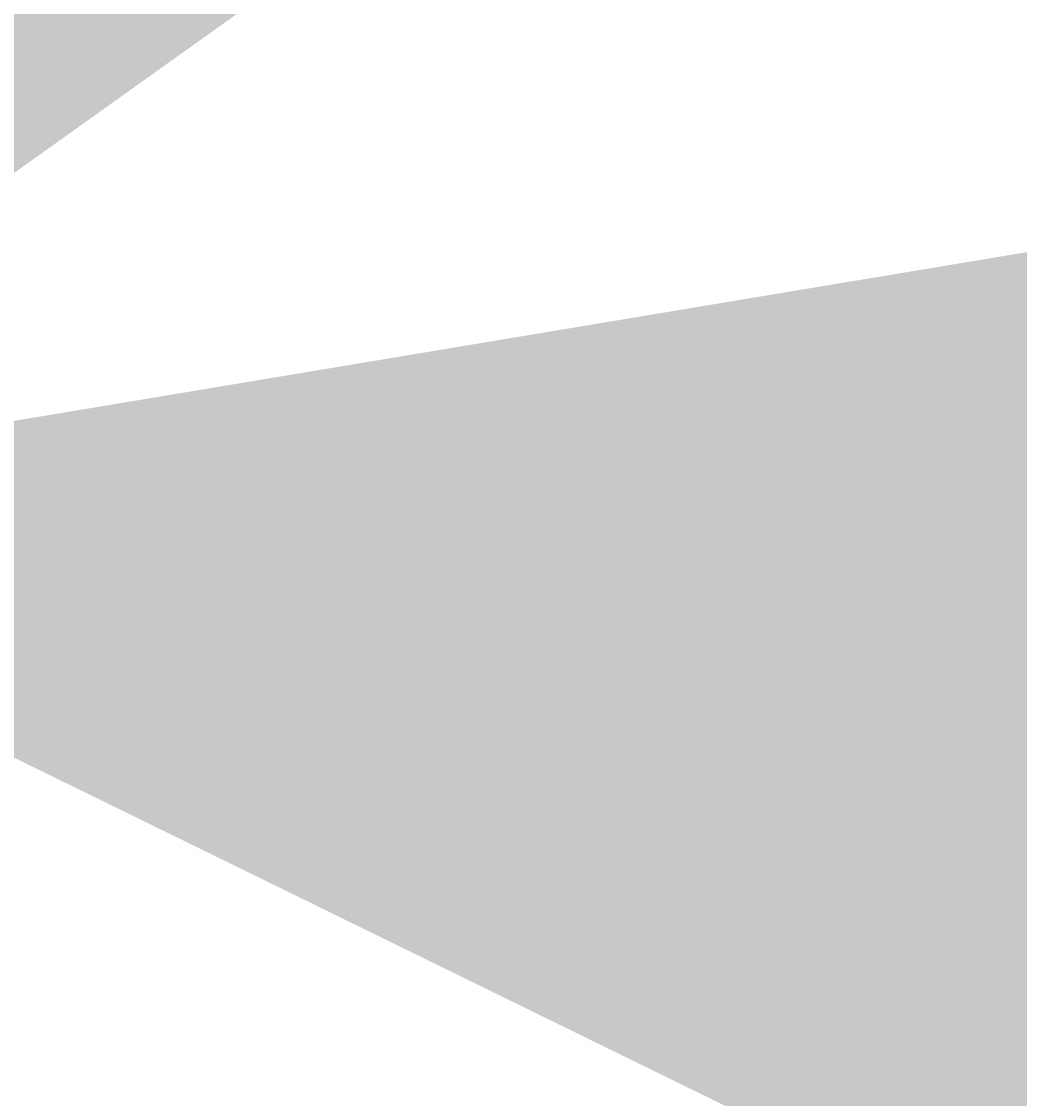
# Model space of a CAD drawing. Units: millimetres. Extents: x -22994 to 29398, y -19990 to 20176.
# Tile 131 of 135: x 2052 to 5745, y -1986 to 2002. Entities that reach past the tile are written whole.
import ezdxf

# ---------------------------------------------------------------- set-up
doc = ezdxf.new("R2010")
doc.units = ezdxf.units.MM
doc.header["$MEASUREMENT"] = 0
doc.layers.add('M-DIMS', color=2, linetype='Continuous', lineweight=18)
doc.styles.get("Standard").update_dxf_attribs({"font": 'arial.ttf'})
doc.dimstyles.get("Standard").update_dxf_attribs({"dimtxt": 0.18, "dimasz": 10000, "dimexe": 0.18, "dimexo": 0.0625, "dimgap": 0.09, "dimtad": 0, "dimtih": 1, "dimtoh": 1, "dimdec": 0, "dimzin": 0, "dimdsep": 46, "dimtxsty": 'Standard', "dimcen": 0.09, "dimadec": 0, "dimazin": 0, "dimtfac": 1, "dimtdec": 0, "dimtofl": 0, "dimtmove": 0, "dimatfit": 3, "dimfxl": 1, "dimtolj": 1, "dimtzin": 0, "dimlwd": 30, "dimarcsym": 0})

# ---------------------------------------------------------------- blocks, each defined once
blk = doc.blocks.new('*D2')
at = {"layer": 'Defpoints', "color": 0, "transparency": 16777216}
for p in [(6.7, 10.3), (290.9, 10.3), (290.9, -5.1)]:
    blk.add_point(p, dxfattribs=at)
at = {"layer": 'M-DIMS', "color": 0, "lineweight": -2, "transparency": 16777216}
for p, q in [((6.7, 10.2), (6.7, -5.3)), ((290.9, 10.2), (290.9, -5.3))]:
    blk.add_line(p, q, dxfattribs=at)
at = {"layer": 'M-DIMS', "color": 0, "lineweight": 30, "transparency": 16777216}
for p, q in [((-9993.3, -5.1), (-19993.3, -5.1)), ((10290.9, -5.1), (20290.9, -5.1))]:
    blk.add_line(p, q, dxfattribs=at)
at = {"layer": 'M-DIMS', "color": 0, "transparency": 16777216}
for points in [[(-9993.3, 1661.6), (-9993.3, -1671.7), (6.7, -5.1)], [(10290.9, 1661.6), (10290.9, -1671.7), (290.9, -5.1)]]:
    blk.add_solid(points, dxfattribs=at)
at = {"layer": 'M-DIMS', "color": 0, "transparency": 16777216, "insert": (148.8, -5.1), "char_height": 0.18, "attachment_point": 5}
blk.add_mtext('\\A1;284.2', dxfattribs=at)
blk = doc.blocks.new('*D3')
at = {"layer": 'Defpoints', "color": 0, "transparency": 16777216}
for p in [(110.3, 204.2), (110.3, 176.4), (95.8, 128)]:
    blk.add_point(p, dxfattribs=at)
at = {"layer": 'M-DIMS', "color": 0, "lineweight": 30, "transparency": 16777216}
for p, q in [((-9904.2, 204.2), (-19904.2, 204.2)), ((10110.3, 204.2), (20110.3, 204.2))]:
    blk.add_line(p, q, dxfattribs=at)
at = {"layer": 'M-DIMS', "color": 0, "lineweight": -2, "transparency": 16777216}
for p, q in [((95.8, 128), (95.8, 204.3)), ((110.3, 176.4), (110.3, 204.3))]:
    blk.add_line(p, q, dxfattribs=at)
at = {"layer": 'M-DIMS', "color": 0, "transparency": 16777216}
for points in [[(-9904.2, 1870.8), (-9904.2, -1462.5), (95.8, 204.2)], [(10110.3, 1870.8), (10110.3, -1462.5), (110.3, 204.2)]]:
    blk.add_solid(points, dxfattribs=at)
at = {"layer": 'M-DIMS', "color": 0, "transparency": 16777216, "insert": (103, 204.2), "char_height": 0.18, "attachment_point": 5}
blk.add_mtext('\\A1;14.432', dxfattribs=at)
blk = doc.blocks.new('*D4')
at = {"layer": 'Defpoints', "color": 0, "transparency": 16777216}
for p in [(116.3, 204.2), (110.3, 176.4), (116.3, 176.4)]:
    blk.add_point(p, dxfattribs=at)
at = {"layer": 'M-DIMS', "color": 0, "lineweight": 30, "transparency": 16777216}
for p, q in [((-9889.7, 204.2), (-19889.7, 204.2)), ((10116.3, 204.2), (20116.3, 204.2))]:
    blk.add_line(p, q, dxfattribs=at)
at = {"layer": 'M-DIMS', "color": 0, "lineweight": -2, "transparency": 16777216}
for p, q in [((110.3, 176.4), (110.3, 204.3)), ((116.3, 176.4), (116.3, 204.3))]:
    blk.add_line(p, q, dxfattribs=at)
at = {"layer": 'M-DIMS', "color": 0, "transparency": 16777216}
for points in [[(-9889.7, 1870.8), (-9889.7, -1462.5), (110.3, 204.2)], [(10116.3, 1870.8), (10116.3, -1462.5), (116.3, 204.2)]]:
    blk.add_solid(points, dxfattribs=at)
at = {"layer": 'M-DIMS', "color": 0, "transparency": 16777216, "insert": (113.3, 204.2), "char_height": 0.18, "attachment_point": 5}
blk.add_mtext('\\A1;6', dxfattribs=at)
blk = doc.blocks.new('*D5')
at = {"layer": 'Defpoints', "color": 0, "transparency": 16777216}
for p in [(181.3, 204.2), (116.3, 176.4), (181.3, 176.4)]:
    blk.add_point(p, dxfattribs=at)
at = {"layer": 'M-DIMS', "color": 0, "lineweight": 30, "transparency": 16777216}
for p, q in [((-9883.7, 204.2), (-19883.7, 204.2)), ((10181.3, 204.2), (20181.3, 204.2))]:
    blk.add_line(p, q, dxfattribs=at)
at = {"layer": 'M-DIMS', "color": 0, "lineweight": -2, "transparency": 16777216}
for p, q in [((116.3, 176.4), (116.3, 204.3)), ((181.3, 176.4), (181.3, 204.3))]:
    blk.add_line(p, q, dxfattribs=at)
at = {"layer": 'M-DIMS', "color": 0, "transparency": 16777216}
for points in [[(-9883.7, 1870.8), (-9883.7, -1462.5), (116.3, 204.2)], [(10181.3, 1870.8), (10181.3, -1462.5), (181.3, 204.2)]]:
    blk.add_solid(points, dxfattribs=at)
at = {"layer": 'M-DIMS', "color": 0, "transparency": 16777216, "insert": (148.8, 204.2), "char_height": 0.18, "attachment_point": 5}
blk.add_mtext('\\A1;65', dxfattribs=at)
blk = doc.blocks.new('*D6')
at = {"layer": 'Defpoints', "color": 0, "transparency": 16777216}
for p in [(187.3, 204.2), (181.3, 176.4), (187.3, 176.4)]:
    blk.add_point(p, dxfattribs=at)
at = {"layer": 'M-DIMS', "color": 0, "lineweight": 30, "transparency": 16777216}
for p, q in [((-9818.7, 204.2), (-19818.7, 204.2)), ((10187.3, 204.2), (20187.3, 204.2))]:
    blk.add_line(p, q, dxfattribs=at)
at = {"layer": 'M-DIMS', "color": 0, "lineweight": -2, "transparency": 16777216}
for p, q in [((181.3, 176.4), (181.3, 204.3)), ((187.3, 176.4), (187.3, 204.3))]:
    blk.add_line(p, q, dxfattribs=at)
at = {"layer": 'M-DIMS', "color": 0, "transparency": 16777216}
for points in [[(-9818.7, 1870.8), (-9818.7, -1462.5), (181.3, 204.2)], [(10187.3, 1870.8), (10187.3, -1462.5), (187.3, 204.2)]]:
    blk.add_solid(points, dxfattribs=at)
at = {"layer": 'M-DIMS', "color": 0, "transparency": 16777216, "insert": (184.3, 204.2), "char_height": 0.18, "attachment_point": 5}
blk.add_mtext('\\A1;6', dxfattribs=at)
blk = doc.blocks.new('*D7')
at = {"layer": 'Defpoints', "color": 0, "transparency": 16777216}
for p in [(201.7, 204.2), (187.3, 176.4), (201.7, 128)]:
    blk.add_point(p, dxfattribs=at)
at = {"layer": 'M-DIMS', "color": 0, "lineweight": 30, "transparency": 16777216}
for p, q in [((-9812.7, 204.2), (-19812.7, 204.2)), ((10201.7, 204.2), (20201.7, 204.2))]:
    blk.add_line(p, q, dxfattribs=at)
at = {"layer": 'M-DIMS', "color": 0, "lineweight": -2, "transparency": 16777216}
for p, q in [((187.3, 176.4), (187.3, 204.3)), ((201.7, 128), (201.7, 204.3))]:
    blk.add_line(p, q, dxfattribs=at)
at = {"layer": 'M-DIMS', "color": 0, "transparency": 16777216}
for points in [[(-9812.7, 1870.8), (-9812.7, -1462.5), (187.3, 204.2)], [(10201.7, 1870.8), (10201.7, -1462.5), (201.7, 204.2)]]:
    blk.add_solid(points, dxfattribs=at)
at = {"layer": 'M-DIMS', "color": 0, "transparency": 16777216, "insert": (194.5, 204.2), "char_height": 0.18, "attachment_point": 5}
blk.add_mtext('\\A1;14.432', dxfattribs=at)
blk = doc.blocks.new('*D8')
at = {"layer": 'Defpoints', "color": 0, "transparency": 16777216}
for p in [(227.6, 204.2), (201.7, 128), (227.6, 146.7)]:
    blk.add_point(p, dxfattribs=at)
at = {"layer": 'M-DIMS', "color": 0, "lineweight": 30, "transparency": 16777216}
for p, q in [((-9798.3, 204.2), (-19798.3, 204.2)), ((10227.6, 204.2), (20227.6, 204.2))]:
    blk.add_line(p, q, dxfattribs=at)
at = {"layer": 'M-DIMS', "color": 0, "lineweight": -2, "transparency": 16777216}
for p, q in [((201.7, 128), (201.7, 204.3)), ((227.6, 146.8), (227.6, 204.3))]:
    blk.add_line(p, q, dxfattribs=at)
at = {"layer": 'M-DIMS', "color": 0, "transparency": 16777216}
for points in [[(-9798.3, 1870.8), (-9798.3, -1462.5), (201.7, 204.2)], [(10227.6, 1870.8), (10227.6, -1462.5), (227.6, 204.2)]]:
    blk.add_solid(points, dxfattribs=at)
at = {"layer": 'M-DIMS', "color": 0, "transparency": 16777216, "insert": (214.7, 204.2), "char_height": 0.18, "attachment_point": 5}
blk.add_mtext('\\A1;25.95', dxfattribs=at)
blk = doc.blocks.new('*D10')
at = {"layer": 'Defpoints', "color": 0, "transparency": 16777216}
for p in [(125.6, 136.1), (133.3, 136.1), (133.3, -5.1)]:
    blk.add_point(p, dxfattribs=at)
at = {"layer": 'M-DIMS', "color": 0, "lineweight": -2, "transparency": 16777216}
for p, q in [((125.6, 136), (125.6, -5.3)), ((133.3, 136), (133.3, -5.3))]:
    blk.add_line(p, q, dxfattribs=at)
at = {"layer": 'M-DIMS', "color": 0, "lineweight": 30, "transparency": 16777216}
for p, q in [((-9874.4, -5.1), (-19874.4, -5.1)), ((10133.3, -5.1), (20133.3, -5.1))]:
    blk.add_line(p, q, dxfattribs=at)
at = {"layer": 'M-DIMS', "color": 0, "transparency": 16777216}
for points in [[(-9874.4, 1661.6), (-9874.4, -1671.7), (125.6, -5.1)], [(10133.3, 1661.6), (10133.3, -1671.7), (133.3, -5.1)]]:
    blk.add_solid(points, dxfattribs=at)
at = {"layer": 'M-DIMS', "color": 0, "transparency": 16777216, "insert": (129.5, -5.1), "char_height": 0.18, "attachment_point": 5}
blk.add_mtext('\\A1;7.696', dxfattribs=at)
blk = doc.blocks.new('*D11')
at = {"layer": 'Defpoints', "color": 0, "transparency": 16777216}
for p in [(133.3, 136.1), (135.6, 136.1), (135.6, -5.1)]:
    blk.add_point(p, dxfattribs=at)
at = {"layer": 'M-DIMS', "color": 0, "lineweight": -2, "transparency": 16777216}
for p, q in [((133.3, 136), (133.3, -5.3)), ((135.6, 136), (135.6, -5.3))]:
    blk.add_line(p, q, dxfattribs=at)
at = {"layer": 'M-DIMS', "color": 0, "lineweight": 30, "transparency": 16777216}
for p, q in [((-9866.7, -5.1), (-19866.7, -5.1)), ((10135.6, -5.1), (20135.6, -5.1))]:
    blk.add_line(p, q, dxfattribs=at)
at = {"layer": 'M-DIMS', "color": 0, "transparency": 16777216}
for points in [[(-9866.7, 1661.6), (-9866.7, -1671.7), (133.3, -5.1)], [(10135.6, 1661.6), (10135.6, -1671.7), (135.6, -5.1)]]:
    blk.add_solid(points, dxfattribs=at)
at = {"layer": 'M-DIMS', "color": 0, "transparency": 16777216, "insert": (134.5, -5.1), "char_height": 0.18, "attachment_point": 5}
blk.add_mtext('\\A1;2.304', dxfattribs=at)
blk = doc.blocks.new('*D12')
at = {"layer": 'Defpoints', "color": 0, "transparency": 16777216}
for p in [(135.6, 136.1), (145.6, 136.1), (145.6, -5.1)]:
    blk.add_point(p, dxfattribs=at)
at = {"layer": 'M-DIMS', "color": 0, "lineweight": -2, "transparency": 16777216}
for p, q in [((135.6, 136), (135.6, -5.3)), ((145.6, 136), (145.6, -5.3))]:
    blk.add_line(p, q, dxfattribs=at)
at = {"layer": 'M-DIMS', "color": 0, "lineweight": 30, "transparency": 16777216}
for p, q in [((-9864.4, -5.1), (-19864.4, -5.1)), ((10145.6, -5.1), (20145.6, -5.1))]:
    blk.add_line(p, q, dxfattribs=at)
at = {"layer": 'M-DIMS', "color": 0, "transparency": 16777216}
for points in [[(-9864.4, 1661.6), (-9864.4, -1671.7), (135.6, -5.1)], [(10145.6, 1661.6), (10145.6, -1671.7), (145.6, -5.1)]]:
    blk.add_solid(points, dxfattribs=at)
at = {"layer": 'M-DIMS', "color": 0, "transparency": 16777216, "insert": (140.6, -5.1), "char_height": 0.18, "attachment_point": 5}
blk.add_mtext('\\A1;10', dxfattribs=at)
blk = doc.blocks.new('*D13')
at = {"layer": 'Defpoints', "color": 0, "transparency": 16777216}
for p in [(145.6, 136.1), (155.6, 136.1), (155.6, -5.1)]:
    blk.add_point(p, dxfattribs=at)
at = {"layer": 'M-DIMS', "color": 0, "lineweight": -2, "transparency": 16777216}
for p, q in [((145.6, 136), (145.6, -5.3)), ((155.6, 136), (155.6, -5.3))]:
    blk.add_line(p, q, dxfattribs=at)
at = {"layer": 'M-DIMS', "color": 0, "lineweight": 30, "transparency": 16777216}
for p, q in [((-9854.4, -5.1), (-19854.4, -5.1)), ((10155.6, -5.1), (20155.6, -5.1))]:
    blk.add_line(p, q, dxfattribs=at)
at = {"layer": 'M-DIMS', "color": 0, "transparency": 16777216}
for points in [[(-9854.4, 1661.6), (-9854.4, -1671.7), (145.6, -5.1)], [(10155.6, 1661.6), (10155.6, -1671.7), (155.6, -5.1)]]:
    blk.add_solid(points, dxfattribs=at)
at = {"layer": 'M-DIMS', "color": 0, "transparency": 16777216, "insert": (150.6, -5.1), "char_height": 0.18, "attachment_point": 5}
blk.add_mtext('\\A1;10', dxfattribs=at)
blk = doc.blocks.new('*D14')
at = {"layer": 'Defpoints', "color": 0, "transparency": 16777216}
for p in [(155.6, 136.1), (165.6, 136.1), (165.6, -5.1)]:
    blk.add_point(p, dxfattribs=at)
at = {"layer": 'M-DIMS', "color": 0, "lineweight": -2, "transparency": 16777216}
for p, q in [((155.6, 136), (155.6, -5.3)), ((165.6, 136), (165.6, -5.3))]:
    blk.add_line(p, q, dxfattribs=at)
at = {"layer": 'M-DIMS', "color": 0, "lineweight": 30, "transparency": 16777216}
for p, q in [((-9844.4, -5.1), (-19844.4, -5.1)), ((10165.6, -5.1), (20165.6, -5.1))]:
    blk.add_line(p, q, dxfattribs=at)
at = {"layer": 'M-DIMS', "color": 0, "transparency": 16777216}
for points in [[(-9844.4, 1661.6), (-9844.4, -1671.7), (155.6, -5.1)], [(10165.6, 1661.6), (10165.6, -1671.7), (165.6, -5.1)]]:
    blk.add_solid(points, dxfattribs=at)
at = {"layer": 'M-DIMS', "color": 0, "transparency": 16777216, "insert": (160.6, -5.1), "char_height": 0.18, "attachment_point": 5}
blk.add_mtext('\\A1;10', dxfattribs=at)
blk = doc.blocks.new('*D16')
at = {"layer": 'Defpoints', "color": 0, "transparency": 16777216}
for p in [(120.2, 204.2), (110.5, 48), (120.2, 48)]:
    blk.add_point(p, dxfattribs=at)
at = {"layer": 'M-DIMS', "color": 0, "lineweight": 30, "transparency": 16777216}
for p, q in [((-9889.5, 204.2), (-19889.5, 204.2)), ((10120.2, 204.2), (20120.2, 204.2))]:
    blk.add_line(p, q, dxfattribs=at)
at = {"layer": 'M-DIMS', "color": 0, "lineweight": -2, "transparency": 16777216}
for p, q in [((110.5, 48.1), (110.5, 204.3)), ((120.2, 48.1), (120.2, 204.3))]:
    blk.add_line(p, q, dxfattribs=at)
at = {"layer": 'M-DIMS', "color": 0, "transparency": 16777216}
for points in [[(-9889.5, 1870.8), (-9889.5, -1462.5), (110.5, 204.2)], [(10120.2, 1870.8), (10120.2, -1462.5), (120.2, 204.2)]]:
    blk.add_solid(points, dxfattribs=at)
at = {"layer": 'M-DIMS', "color": 0, "transparency": 16777216, "insert": (115.3, 204.2), "char_height": 0.18, "attachment_point": 5}
blk.add_mtext('\\A1;9.704', dxfattribs=at)
blk = doc.blocks.new('*D17')
at = {"layer": 'Defpoints', "color": 0, "transparency": 16777216}
for p in [(126.2, 204.2), (120.2, 48), (126.2, 48)]:
    blk.add_point(p, dxfattribs=at)
at = {"layer": 'M-DIMS', "color": 0, "lineweight": 30, "transparency": 16777216}
for p, q in [((-9879.8, 204.2), (-19879.8, 204.2)), ((10126.2, 204.2), (20126.2, 204.2))]:
    blk.add_line(p, q, dxfattribs=at)
at = {"layer": 'M-DIMS', "color": 0, "lineweight": -2, "transparency": 16777216}
for p, q in [((120.2, 48.1), (120.2, 204.3)), ((126.2, 48.1), (126.2, 204.3))]:
    blk.add_line(p, q, dxfattribs=at)
at = {"layer": 'M-DIMS', "color": 0, "transparency": 16777216}
for points in [[(-9879.8, 1870.8), (-9879.8, -1462.5), (120.2, 204.2)], [(10126.2, 1870.8), (10126.2, -1462.5), (126.2, 204.2)]]:
    blk.add_solid(points, dxfattribs=at)
at = {"layer": 'M-DIMS', "color": 0, "transparency": 16777216, "insert": (123.2, 204.2), "char_height": 0.18, "attachment_point": 5}
blk.add_mtext('\\A1;6', dxfattribs=at)
blk = doc.blocks.new('*D18')
at = {"layer": 'Defpoints', "color": 0, "transparency": 16777216}
for p in [(132.2, 204.2), (126.2, 48), (132.2, 48)]:
    blk.add_point(p, dxfattribs=at)
at = {"layer": 'M-DIMS', "color": 0, "lineweight": 30, "transparency": 16777216}
for p, q in [((-9873.8, 204.2), (-19873.8, 204.2)), ((10132.2, 204.2), (20132.2, 204.2))]:
    blk.add_line(p, q, dxfattribs=at)
at = {"layer": 'M-DIMS', "color": 0, "lineweight": -2, "transparency": 16777216}
for p, q in [((126.2, 48.1), (126.2, 204.3)), ((132.2, 48.1), (132.2, 204.3))]:
    blk.add_line(p, q, dxfattribs=at)
at = {"layer": 'M-DIMS', "color": 0, "transparency": 16777216}
for points in [[(-9873.8, 1870.8), (-9873.8, -1462.5), (126.2, 204.2)], [(10132.2, 1870.8), (10132.2, -1462.5), (132.2, 204.2)]]:
    blk.add_solid(points, dxfattribs=at)
at = {"layer": 'M-DIMS', "color": 0, "transparency": 16777216, "insert": (129.2, 204.2), "char_height": 0.18, "attachment_point": 5}
blk.add_mtext('\\A1;6', dxfattribs=at)
blk = doc.blocks.new('*D19')
at = {"layer": 'Defpoints', "color": 0, "transparency": 16777216}
for p in [(138.2, 204.2), (132.2, 48), (138.2, 48)]:
    blk.add_point(p, dxfattribs=at)
at = {"layer": 'M-DIMS', "color": 0, "lineweight": 30, "transparency": 16777216}
for p, q in [((-9867.8, 204.2), (-19867.8, 204.2)), ((10138.2, 204.2), (20138.2, 204.2))]:
    blk.add_line(p, q, dxfattribs=at)
at = {"layer": 'M-DIMS', "color": 0, "lineweight": -2, "transparency": 16777216}
for p, q in [((132.2, 48.1), (132.2, 204.3)), ((138.2, 48.1), (138.2, 204.3))]:
    blk.add_line(p, q, dxfattribs=at)
at = {"layer": 'M-DIMS', "color": 0, "transparency": 16777216}
for points in [[(-9867.8, 1870.8), (-9867.8, -1462.5), (132.2, 204.2)], [(10138.2, 1870.8), (10138.2, -1462.5), (138.2, 204.2)]]:
    blk.add_solid(points, dxfattribs=at)
at = {"layer": 'M-DIMS', "color": 0, "transparency": 16777216, "insert": (135.2, 204.2), "char_height": 0.18, "attachment_point": 5}
blk.add_mtext('\\A1;6', dxfattribs=at)
blk = doc.blocks.new('*D20')
at = {"layer": 'Defpoints', "color": 0, "transparency": 16777216}
for p in [(144.2, 204.2), (138.2, 48), (144.2, 48)]:
    blk.add_point(p, dxfattribs=at)
at = {"layer": 'M-DIMS', "color": 0, "lineweight": 30, "transparency": 16777216}
for p, q in [((-9861.8, 204.2), (-19861.8, 204.2)), ((10144.2, 204.2), (20144.2, 204.2))]:
    blk.add_line(p, q, dxfattribs=at)
at = {"layer": 'M-DIMS', "color": 0, "lineweight": -2, "transparency": 16777216}
for p, q in [((138.2, 48.1), (138.2, 204.3)), ((144.2, 48.1), (144.2, 204.3))]:
    blk.add_line(p, q, dxfattribs=at)
at = {"layer": 'M-DIMS', "color": 0, "transparency": 16777216}
for points in [[(-9861.8, 1870.8), (-9861.8, -1462.5), (138.2, 204.2)], [(10144.2, 1870.8), (10144.2, -1462.5), (144.2, 204.2)]]:
    blk.add_solid(points, dxfattribs=at)
at = {"layer": 'M-DIMS', "color": 0, "transparency": 16777216, "insert": (141.2, 204.2), "char_height": 0.18, "attachment_point": 5}
blk.add_mtext('\\A1;6', dxfattribs=at)
blk = doc.blocks.new('*D21')
at = {"layer": 'Defpoints', "color": 0, "transparency": 16777216}
for p in [(149.1, 204.2), (144.2, 48), (149.1, 48)]:
    blk.add_point(p, dxfattribs=at)
at = {"layer": 'M-DIMS', "color": 0, "lineweight": 30, "transparency": 16777216}
for p, q in [((-9855.8, 204.2), (-19855.8, 204.2)), ((10149.1, 204.2), (20149.1, 204.2))]:
    blk.add_line(p, q, dxfattribs=at)
at = {"layer": 'M-DIMS', "color": 0, "lineweight": -2, "transparency": 16777216}
for p, q in [((144.2, 48.1), (144.2, 204.3)), ((149.1, 48.1), (149.1, 204.3))]:
    blk.add_line(p, q, dxfattribs=at)
at = {"layer": 'M-DIMS', "color": 0, "transparency": 16777216}
for points in [[(-9855.8, 1870.8), (-9855.8, -1462.5), (144.2, 204.2)], [(10149.1, 1870.8), (10149.1, -1462.5), (149.1, 204.2)]]:
    blk.add_solid(points, dxfattribs=at)
at = {"layer": 'M-DIMS', "color": 0, "transparency": 16777216, "insert": (146.6, 204.2), "char_height": 0.18, "attachment_point": 5}
blk.add_mtext('\\A1;4.945', dxfattribs=at)
blk = doc.blocks.new('*D22')
at = {"layer": 'Defpoints', "color": 0, "transparency": 16777216}
for p in [(149.1, 31), (155.1, 31), (155.1, -5.1)]:
    blk.add_point(p, dxfattribs=at)
at = {"layer": 'M-DIMS', "color": 0, "lineweight": -2, "transparency": 16777216}
for p, q in [((149.1, 30.9), (149.1, -5.3)), ((155.1, 30.9), (155.1, -5.3))]:
    blk.add_line(p, q, dxfattribs=at)
at = {"layer": 'M-DIMS', "color": 0, "lineweight": 30, "transparency": 16777216}
for p, q in [((-9850.9, -5.1), (-19850.9, -5.1)), ((10155.1, -5.1), (20155.1, -5.1))]:
    blk.add_line(p, q, dxfattribs=at)
at = {"layer": 'M-DIMS', "color": 0, "transparency": 16777216}
for points in [[(-9850.9, 1661.6), (-9850.9, -1671.7), (149.1, -5.1)], [(10155.1, 1661.6), (10155.1, -1671.7), (155.1, -5.1)]]:
    blk.add_solid(points, dxfattribs=at)
at = {"layer": 'M-DIMS', "color": 0, "transparency": 16777216, "insert": (152.1, -5.1), "char_height": 0.18, "attachment_point": 5}
blk.add_mtext('\\A1;6', dxfattribs=at)
blk = doc.blocks.new('*D23')
at = {"layer": 'Defpoints', "color": 0, "transparency": 16777216}
for p in [(155.1, 31), (161.1, 31), (161.1, -5.1)]:
    blk.add_point(p, dxfattribs=at)
at = {"layer": 'M-DIMS', "color": 0, "lineweight": -2, "transparency": 16777216}
for p, q in [((155.1, 30.9), (155.1, -5.3)), ((161.1, 30.9), (161.1, -5.3))]:
    blk.add_line(p, q, dxfattribs=at)
at = {"layer": 'M-DIMS', "color": 0, "lineweight": 30, "transparency": 16777216}
for p, q in [((-9844.9, -5.1), (-19844.9, -5.1)), ((10161.1, -5.1), (20161.1, -5.1))]:
    blk.add_line(p, q, dxfattribs=at)
at = {"layer": 'M-DIMS', "color": 0, "transparency": 16777216}
for points in [[(-9844.9, 1661.6), (-9844.9, -1671.7), (155.1, -5.1)], [(10161.1, 1661.6), (10161.1, -1671.7), (161.1, -5.1)]]:
    blk.add_solid(points, dxfattribs=at)
at = {"layer": 'M-DIMS', "color": 0, "transparency": 16777216, "insert": (158.1, -5.1), "char_height": 0.18, "attachment_point": 5}
blk.add_mtext('\\A1;6', dxfattribs=at)
blk = doc.blocks.new('*D24')
at = {"layer": 'Defpoints', "color": 0, "transparency": 16777216}
for p in [(161.1, 31), (166.4, 31), (166.4, -5.1)]:
    blk.add_point(p, dxfattribs=at)
at = {"layer": 'M-DIMS', "color": 0, "lineweight": -2, "transparency": 16777216}
for p, q in [((161.1, 30.9), (161.1, -5.3)), ((166.4, 30.9), (166.4, -5.3))]:
    blk.add_line(p, q, dxfattribs=at)
at = {"layer": 'M-DIMS', "color": 0, "lineweight": 30, "transparency": 16777216}
for p, q in [((-9838.9, -5.1), (-19838.9, -5.1)), ((10166.4, -5.1), (20166.4, -5.1))]:
    blk.add_line(p, q, dxfattribs=at)
at = {"layer": 'M-DIMS', "color": 0, "transparency": 16777216}
for points in [[(-9838.9, 1661.6), (-9838.9, -1671.7), (161.1, -5.1)], [(10166.4, 1661.6), (10166.4, -1671.7), (166.4, -5.1)]]:
    blk.add_solid(points, dxfattribs=at)
at = {"layer": 'M-DIMS', "color": 0, "transparency": 16777216, "insert": (163.8, -5.1), "char_height": 0.18, "attachment_point": 5}
blk.add_mtext('\\A1;5.323', dxfattribs=at)
blk = doc.blocks.new('*D25')
at = {"layer": 'Defpoints', "color": 0, "transparency": 16777216}
for p in [(166.4, 31), (172.4, 31), (172.4, -5.1)]:
    blk.add_point(p, dxfattribs=at)
at = {"layer": 'M-DIMS', "color": 0, "lineweight": -2, "transparency": 16777216}
for p, q in [((166.4, 30.9), (166.4, -5.3)), ((172.4, 30.9), (172.4, -5.3))]:
    blk.add_line(p, q, dxfattribs=at)
at = {"layer": 'M-DIMS', "color": 0, "lineweight": 30, "transparency": 16777216}
for p, q in [((-9833.6, -5.1), (-19833.6, -5.1)), ((10172.4, -5.1), (20172.4, -5.1))]:
    blk.add_line(p, q, dxfattribs=at)
at = {"layer": 'M-DIMS', "color": 0, "transparency": 16777216}
for points in [[(-9833.6, 1661.6), (-9833.6, -1671.7), (166.4, -5.1)], [(10172.4, 1661.6), (10172.4, -1671.7), (172.4, -5.1)]]:
    blk.add_solid(points, dxfattribs=at)
at = {"layer": 'M-DIMS', "color": 0, "transparency": 16777216, "insert": (169.4, -5.1), "char_height": 0.18, "attachment_point": 5}
blk.add_mtext('\\A1;6', dxfattribs=at)
blk = doc.blocks.new('*D26')
at = {"layer": 'Defpoints', "color": 0, "transparency": 16777216}
for p in [(172.4, 31), (178.4, 31), (178.4, -5.1)]:
    blk.add_point(p, dxfattribs=at)
at = {"layer": 'M-DIMS', "color": 0, "lineweight": -2, "transparency": 16777216}
for p, q in [((172.4, 30.9), (172.4, -5.3)), ((178.4, 30.9), (178.4, -5.3))]:
    blk.add_line(p, q, dxfattribs=at)
at = {"layer": 'M-DIMS', "color": 0, "lineweight": 30, "transparency": 16777216}
for p, q in [((-9827.6, -5.1), (-19827.6, -5.1)), ((10178.4, -5.1), (20178.4, -5.1))]:
    blk.add_line(p, q, dxfattribs=at)
at = {"layer": 'M-DIMS', "color": 0, "transparency": 16777216}
for points in [[(-9827.6, 1661.6), (-9827.6, -1671.7), (172.4, -5.1)], [(10178.4, 1661.6), (10178.4, -1671.7), (178.4, -5.1)]]:
    blk.add_solid(points, dxfattribs=at)
at = {"layer": 'M-DIMS', "color": 0, "transparency": 16777216, "insert": (175.4, -5.1), "char_height": 0.18, "attachment_point": 5}
blk.add_mtext('\\A1;6', dxfattribs=at)
blk = doc.blocks.new('*D27')
at = {"layer": 'Defpoints', "color": 0, "transparency": 16777216}
for p in [(178.4, 31), (188.1, 31), (188.1, -5.1)]:
    blk.add_point(p, dxfattribs=at)
at = {"layer": 'M-DIMS', "color": 0, "lineweight": -2, "transparency": 16777216}
for p, q in [((178.4, 30.9), (178.4, -5.3)), ((188.1, 30.9), (188.1, -5.3))]:
    blk.add_line(p, q, dxfattribs=at)
at = {"layer": 'M-DIMS', "color": 0, "lineweight": 30, "transparency": 16777216}
for p, q in [((-9821.6, -5.1), (-19821.6, -5.1)), ((10188.1, -5.1), (20188.1, -5.1))]:
    blk.add_line(p, q, dxfattribs=at)
at = {"layer": 'M-DIMS', "color": 0, "transparency": 16777216}
for points in [[(-9821.6, 1661.6), (-9821.6, -1671.7), (178.4, -5.1)], [(10188.1, 1661.6), (10188.1, -1671.7), (188.1, -5.1)]]:
    blk.add_solid(points, dxfattribs=at)
at = {"layer": 'M-DIMS', "color": 0, "transparency": 16777216, "insert": (183.3, -5.1), "char_height": 0.18, "attachment_point": 5}
blk.add_mtext('\\A1;9.679', dxfattribs=at)
blk = doc.blocks.new('*D29')
at = {"layer": 'Defpoints', "color": 0, "transparency": 16777216}
for p in [(36.8, 80), (64, 80)]:
    blk.add_point(p, dxfattribs=at)
at = {"layer": 'M-DIMS', "color": 0, "lineweight": -2, "transparency": 16777216}
for p, q in [((50.3, 80), (50.5, 80)), ((50.4, 80), (50.4, 80.1))]:
    blk.add_line(p, q, dxfattribs=at)
at = {"layer": 'M-DIMS', "color": 0, "lineweight": 30, "transparency": 16777216}
blk.add_line((20064, 80), (10064, 80), dxfattribs=at)
at = {"layer": 'M-DIMS', "color": 0, "transparency": 16777216}
blk.add_solid([(10064, 1746.7), (10064, -1586.6), (64, 80)], dxfattribs=at)
at = {"layer": 'M-DIMS', "color": 0, "transparency": 16777216, "insert": (20064.5, 80), "char_height": 0.18, "attachment_point": 5}
blk.add_mtext('\\A1;∅27.23', dxfattribs=at)
blk = doc.blocks.new('*D30')
at = {"layer": 'Defpoints', "color": 0, "transparency": 16777216}
for p in [(216.3, 146.7), (239, 146.7)]:
    blk.add_point(p, dxfattribs=at)
at = {"layer": 'M-DIMS', "color": 0, "lineweight": -2, "transparency": 16777216}
for p, q in [((227.6, 146.6), (227.6, 146.8)), ((227.6, 146.7), (227.7, 146.7))]:
    blk.add_line(p, q, dxfattribs=at)
at = {"layer": 'M-DIMS', "color": 0, "lineweight": 30, "transparency": 16777216}
blk.add_line((20239, 147.5), (10239, 147.1), dxfattribs=at)
at = {"layer": 'M-DIMS', "color": 0, "transparency": 16777216}
blk.add_solid([(10238.9, 1813.8), (10239, -1519.6), (239, 146.7)], dxfattribs=at)
at = {"layer": 'M-DIMS', "color": 0, "transparency": 16777216, "insert": (20239.5, 147.5), "char_height": 0.18, "attachment_point": 5}
blk.add_mtext('\\A1;∅22.667', dxfattribs=at)
blk = doc.blocks.new('*D31')
at = {"layer": 'Defpoints', "color": 0, "transparency": 16777216}
for p in [(223.2, 146.7), (232.1, 146.7)]:
    blk.add_point(p, dxfattribs=at)
at = {"layer": 'M-DIMS', "color": 0, "lineweight": -2, "transparency": 16777216}
for p, q in [((227.6, 146.6), (227.6, 146.8)), ((227.6, 146.7), (227.7, 146.7))]:
    blk.add_line(p, q, dxfattribs=at)
at = {"layer": 'M-DIMS', "color": 0, "lineweight": 30, "transparency": 16777216}
blk.add_line((20232.1, 148.7), (10232.1, 147.7), dxfattribs=at)
at = {"layer": 'M-DIMS', "color": 0, "transparency": 16777216}
blk.add_solid([(10232, 1814.4), (10232.3, -1519), (232.1, 146.7)], dxfattribs=at)
at = {"layer": 'M-DIMS', "color": 0, "transparency": 16777216, "insert": (20232.6, 148.7), "char_height": 0.18, "attachment_point": 5}
blk.add_mtext('\\A1;∅8.969', dxfattribs=at)
blk = doc.blocks.new('*D33')
at = {"layer": 'Defpoints', "color": 0, "transparency": 16777216}
for p in [(229.6, 154.4), (233, 153.4)]:
    blk.add_point(p, dxfattribs=at)
at = {"layer": 'M-DIMS', "color": 0, "lineweight": -2, "transparency": 16777216}
for p, q in [((229.5, 154.4), (229.7, 154.4)), ((229.6, 154.3), (229.6, 154.5))]:
    blk.add_line(p, q, dxfattribs=at)
at = {"layer": 'M-DIMS', "color": 0, "lineweight": 30, "transparency": 16777216}
for p, q in [((19396.3, -5570.8), (9814.7, -2708.7)), ((29396.3, -5570.8), (19396.3, -5570.8))]:
    blk.add_line(p, q, dxfattribs=at)
at = {"layer": 'M-DIMS', "color": 0, "transparency": 16777216}
blk.add_solid([(10291.7, -1111.8), (9337.7, -4305.7), (233, 153.4)], dxfattribs=at)
at = {"layer": 'M-DIMS', "color": 0, "transparency": 16777216, "insert": (29397, -5570.8), "char_height": 0.18, "attachment_point": 5}
blk.add_mtext('\\A1;6X R3.586', dxfattribs=at)
blk = doc.blocks.new('*D34')
at = {"layer": 'Defpoints', "color": 0, "transparency": 16777216}
for p in [(176.8, 121.1), (178.6, 122.9)]:
    blk.add_point(p, dxfattribs=at)
at = {"layer": 'M-DIMS', "color": 0, "lineweight": 30, "transparency": 16777216}
for p, q in [((14322.4, 14263.3), (7250.5, 7193.1)), ((24322.4, 14263.3), (14322.4, 14263.3))]:
    blk.add_line(p, q, dxfattribs=at)
at = {"layer": 'M-DIMS', "color": 0, "lineweight": -2, "transparency": 16777216}
for p, q in [((176.7, 121.1), (176.9, 121.1)), ((176.8, 121), (176.8, 121.2))]:
    blk.add_line(p, q, dxfattribs=at)
at = {"layer": 'M-DIMS', "color": 0, "transparency": 16777216}
blk.add_solid([(6072.1, 8371.8), (8428.9, 6014.4), (178.6, 122.9)], dxfattribs=at)
at = {"layer": 'M-DIMS', "color": 0, "transparency": 16777216, "insert": (24323, 14263.3), "char_height": 0.18, "attachment_point": 5}
blk.add_mtext('\\A1;6X R2.5', dxfattribs=at)
blk = doc.blocks.new('*D36')
at = {"layer": 'Defpoints', "color": 0, "transparency": 16777216}
for p in [(46.4, 31.3), (46.4, 26.6)]:
    blk.add_point(p, dxfattribs=at)
at = {"layer": 'M-DIMS', "color": 0, "lineweight": 30, "transparency": 16777216}
for p, q in [((57.1, 20031.3), (51.8, 10031.3)), ((10057.1, 20031.3), (57.1, 20031.3))]:
    blk.add_line(p, q, dxfattribs=at)
at = {"layer": 'M-DIMS', "color": 0, "lineweight": -2, "transparency": 16777216}
for p, q in [((46.3, 28.9), (46.5, 28.9)), ((46.4, 28.9), (46.4, 29))]:
    blk.add_line(p, q, dxfattribs=at)
at = {"layer": 'M-DIMS', "color": 0, "transparency": 16777216}
blk.add_solid([(-1614.9, 10032.2), (1718.4, 10030.4), (46.4, 31.3)], dxfattribs=at)
at = {"layer": 'M-DIMS', "color": 0, "transparency": 16777216, "insert": (10057.6, 20031.3), "char_height": 0.18, "attachment_point": 5}
blk.add_mtext('\\A1;∅4.71', dxfattribs=at)
blk = doc.blocks.new('*D37')
at = {"layer": 'Defpoints', "color": 0, "transparency": 16777216}
for p in [(54.8, 118.6), (59.5, 118.6)]:
    blk.add_point(p, dxfattribs=at)
at = {"layer": 'M-DIMS', "color": 0, "lineweight": -2, "transparency": 16777216}
for p, q in [((57.1, 118.6), (57.3, 118.6)), ((57.2, 118.5), (57.2, 118.7))]:
    blk.add_line(p, q, dxfattribs=at)
at = {"layer": 'M-DIMS', "color": 0, "lineweight": 30, "transparency": 16777216}
blk.add_line((20059.5, 116.3), (10059.5, 117.4), dxfattribs=at)
at = {"layer": 'M-DIMS', "color": 0, "transparency": 16777216}
blk.add_solid([(10059.7, 1784.1), (10059.3, -1549.2), (59.5, 118.6)], dxfattribs=at)
at = {"layer": 'M-DIMS', "color": 0, "transparency": 16777216, "insert": (20060, 116.3), "char_height": 0.18, "attachment_point": 5}
blk.add_mtext('\\A1;∅4.659', dxfattribs=at)

msp = doc.modelspace()

# ---------------------------------------------------------------- dimensions: what is measured, and where the dimension line sits
at = {"layer": 'M-DIMS'}
for p1, p2, override, picture, middle in [((46.3875, 26.5934), (46.39, 31.3035), {"dimdec": 2, "dimlfac": 1, "dimrnd": 0, "dimzin": 0, "dimdsep": 46, "dimlunit": 2}, '*D36', (10057.5542, 20031.3006)), ((216.3148, 146.7291), (238.9821, 146.73), {"dimdec": 3, "dimlfac": 1, "dimrnd": 0, "dimzin": 0, "dimdsep": 46, "dimlunit": 2}, '*D30', (20238.9821, 147.4959)), ((223.1641, 146.7291), (232.1328, 146.73), {"dimdec": 3, "dimlfac": 1, "dimrnd": 0, "dimzin": 0, "dimdsep": 46, "dimlunit": 2}, '*D31', (20232.1327, 148.6656))]:
    dim = msp.add_diameter_dim_2p(p1=p1, p2=p2, dimstyle='Standard', override=override, dxfattribs=at)
    dim.commit()
    dim.dimension.update_dxf_attribs({"geometry": picture, "text_midpoint": middle, "dimtype": 163})
for center, mpoint, override, picture, middle in [((176.8123, 121.1277), (178.5802, 122.8952), {"dimdec": 1, "dimlfac": 1, "dimrnd": 0, "dimzin": 0, "dimdsep": 46, "dimlunit": 2}, '*D34', (24322.9703, 14263.3108)), ((229.5613, 154.3773), (232.9972, 153.3509), {"dimdec": 3, "dimlfac": 1, "dimrnd": 0, "dimzin": 0, "dimdsep": 46, "dimlunit": 2}, '*D33', (29397.0125, -5570.8378))]:
    dim = msp.add_radius_dim(center=center, mpoint=mpoint, text='6X <>', dimstyle='Standard', override=override, dxfattribs=at)
    dim.commit()
    dim.dimension.update_dxf_attribs({"geometry": picture, "text_midpoint": middle})
for base, p1, p2, override, picture, middle in [((110.2647, 204.1654), (95.8327, 127.967), (110.2647, 176.3662), {"dimdec": 3, "dimlfac": 1, "dimrnd": 0, "dimzin": 0, "dimdsep": 46, "dimlunit": 2}, '*D3', (103.0487, 204.1654)), ((116.2647, 204.1654), (110.2647, 176.3662), (116.2647, 176.3662), {"dimdec": 0, "dimlfac": 1, "dimrnd": 0, "dimzin": 0, "dimdsep": 46, "dimlunit": 2}, '*D4', (113.2647, 204.1654)), ((120.1702, 204.1654), (110.4658, 48.0349), (120.1702, 48.0349), {"dimdec": 3, "dimlfac": 1, "dimrnd": 0, "dimzin": 0, "dimdsep": 46, "dimlunit": 2}, '*D16', (115.318, 204.1654)), ((181.2647, 204.1654), (116.2647, 176.3662), (181.2647, 176.3662), {"dimdec": 0, "dimlfac": 1, "dimrnd": 0, "dimzin": 0, "dimdsep": 46, "dimlunit": 2}, '*D5', (148.7647, 204.1654)), ((126.1702, 204.1654), (120.1702, 48.0349), (126.1702, 48.0349), {"dimdec": 0, "dimlfac": 1, "dimrnd": 0, "dimzin": 0, "dimdsep": 46, "dimlunit": 2}, '*D17', (123.1702, 204.1654)), ((132.1702, 204.1654), (126.1702, 48.0349), (132.1702, 48.0349), {"dimdec": 0, "dimlfac": 1, "dimrnd": 0, "dimzin": 0, "dimdsep": 46, "dimlunit": 2}, '*D18', (129.1702, 204.1654)), ((138.1702, 204.1654), (132.1702, 48.0349), (138.1702, 48.0349), {"dimdec": 0, "dimlfac": 1, "dimrnd": 0, "dimzin": 0, "dimdsep": 46, "dimlunit": 2}, '*D19', (135.1702, 204.1654)), ((144.1702, 204.1654), (138.1702, 48.0349), (144.1702, 48.0349), {"dimdec": 0, "dimlfac": 1, "dimrnd": 0, "dimzin": 0, "dimdsep": 46, "dimlunit": 2}, '*D20', (141.1702, 204.1654)), ((149.11567, 204.16539), (144.17023, 48.03494), (149.11567, 48.03494), {"dimdec": 3, "dimlfac": 1, "dimrnd": 0, "dimzin": 0, "dimdsep": 46, "dimlunit": 2}, '*D21', (146.64295, 204.16539)), ((187.2647, 204.1654), (181.2647, 176.3662), (187.2647, 176.3662), {"dimdec": 0, "dimlfac": 1, "dimrnd": 0, "dimzin": 0, "dimdsep": 46, "dimlunit": 2}, '*D6', (184.2647, 204.1654)), ((201.6967, 204.1654), (187.2647, 176.3662), (201.6967, 127.967), {"dimdec": 3, "dimlfac": 1, "dimrnd": 0, "dimzin": 0, "dimdsep": 46, "dimlunit": 2}, '*D7', (194.4807, 204.1654)), ((227.6485, 204.1654), (201.6967, 127.967), (227.6485, 146.7296), {"dimdec": 2, "dimlfac": 1, "dimrnd": 0, "dimzin": 0, "dimdsep": 46, "dimlunit": 2}, '*D8', (214.6726, 204.1654)), ((290.852, -5.0787), (6.6773, 10.2713), (290.852, 10.2713), {"dimdec": 1, "dimlfac": 1, "dimrnd": 0, "dimzin": 0, "dimdsep": 46, "dimlunit": 2}, '*D2', (148.7647, -5.0787)), ((133.3459, -5.0787), (125.6498, 136.0713), (133.3459, 136.0713), {"dimdec": 3, "dimlfac": 1, "dimrnd": 0, "dimzin": 0, "dimdsep": 46, "dimlunit": 2}, '*D10', (129.4978, -5.0787)), ((135.6498, -5.0787), (133.3459, 136.0713), (135.6498, 136.0713), {"dimdec": 3, "dimlfac": 1, "dimrnd": 0, "dimzin": 0, "dimdsep": 46, "dimlunit": 2}, '*D11', (134.4978, -5.0787)), ((145.6498, -5.0787), (135.6498, 136.0713), (145.6498, 136.0713), {"dimdec": 0, "dimlfac": 1, "dimrnd": 0, "dimzin": 0, "dimdsep": 46, "dimlunit": 2}, '*D12', (140.6498, -5.0787)), ((155.6498, -5.0787), (145.6498, 136.0713), (155.6498, 136.0713), {"dimdec": 0, "dimlfac": 1, "dimrnd": 0, "dimzin": 0, "dimdsep": 46, "dimlunit": 2}, '*D13', (150.6498, -5.0787)), ((155.1157, -5.0787), (149.1157, 30.9895), (155.1157, 30.9895), {"dimdec": 0, "dimlfac": 1, "dimrnd": 0, "dimzin": 0, "dimdsep": 46, "dimlunit": 2}, '*D22', (152.1157, -5.0787)), ((161.1157, -5.0787), (155.1157, 30.9895), (161.1157, 30.9895), {"dimdec": 0, "dimlfac": 1, "dimrnd": 0, "dimzin": 0, "dimdsep": 46, "dimlunit": 2}, '*D23', (158.1157, -5.0787)), ((165.6498, -5.0787), (155.6498, 136.0713), (165.6498, 136.0713), {"dimdec": 0, "dimlfac": 1, "dimrnd": 0, "dimzin": 0, "dimdsep": 46, "dimlunit": 2}, '*D14', (160.6498, -5.0787)), ((166.4387, -5.0787), (161.1157, 30.9895), (166.4387, 30.9895), {"dimdec": 3, "dimlfac": 1, "dimrnd": 0, "dimzin": 0, "dimdsep": 46, "dimlunit": 2}, '*D24', (163.7772, -5.0787)), ((172.4387, -5.0787), (166.4387, 30.9895), (172.4387, 30.9895), {"dimdec": 0, "dimlfac": 1, "dimrnd": 0, "dimzin": 0, "dimdsep": 46, "dimlunit": 2}, '*D25', (169.4387, -5.0787)), ((178.4387, -5.0787), (172.4387, 30.9895), (178.4387, 30.9895), {"dimdec": 0, "dimlfac": 1, "dimrnd": 0, "dimzin": 0, "dimdsep": 46, "dimlunit": 2}, '*D26', (175.4387, -5.0787)), ((188.1175, -5.0787), (178.4387, 30.9895), (188.1175, 30.9895), {"dimdec": 3, "dimlfac": 1, "dimrnd": 0, "dimzin": 0, "dimdsep": 46, "dimlunit": 2}, '*D27', (183.2781, -5.0787))]:
    dim = msp.add_linear_dim(base=base, p1=p1, p2=p2, dimstyle='Standard', override=override, dxfattribs=at)
    dim.commit()
    dim.dimension.update_dxf_attribs({"geometry": picture, "text_midpoint": middle})
for p1, p2, override, picture, middle in [((54.8343, 118.6145), (59.4936, 118.614), {"dimdec": 3, "dimlfac": 1, "dimrnd": 0, "dimzin": 0, "dimdsep": 46, "dimlunit": 2}, '*D37', (20059.4934, 116.2531)), ((36.8006, 80.045), (64.0296, 80.045), {"dimdec": 2, "dimlfac": 1, "dimrnd": 0, "dimzin": 0, "dimdsep": 46, "dimlunit": 2}, '*D29', (20064.0296, 80.0303))]:
    dim = msp.add_diameter_dim_2p(p1=p1, p2=p2, dimstyle='Standard', override=override, dxfattribs=at)
    dim.commit()
    dim.dimension.update_dxf_attribs({"geometry": picture, "text_midpoint": middle})

doc.saveas('drawing.dxf')
